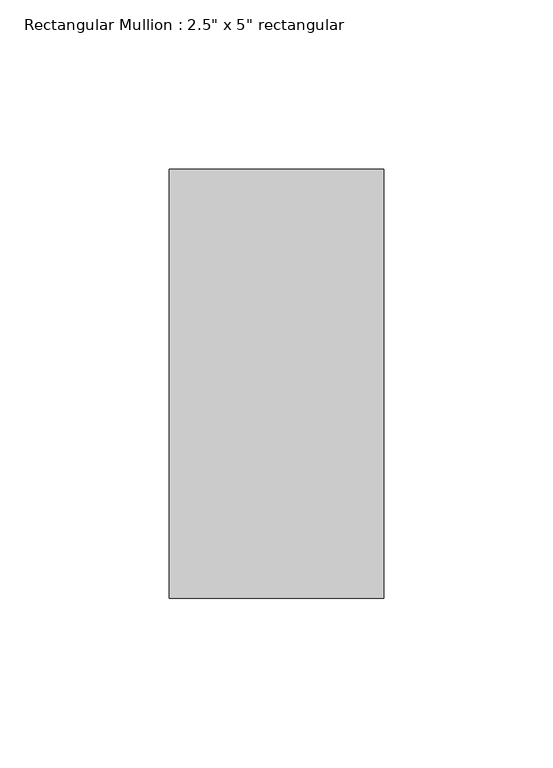
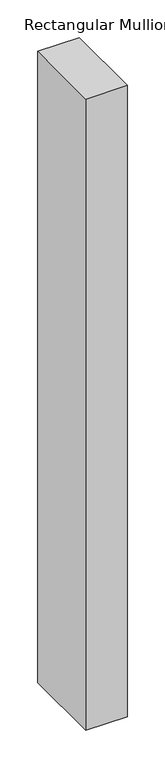
"""IFC4 building model written with IfcOpenShell, lengths in millimetres: member geometry."""

from ifc_helpers import new_model, si_unit, frame, origin, place, context, project, spatial, polyline, outline, extrude, source, transform, mapped, element, save


def member_0bcad3a7(model_context):
    return source(origin(), model_context, "Body", "SweptSolid", [
        extrude(outline(polyline([(0.0, 63.5), (0.0, -63.5), (-63.5, -63.5), (-63.5, 63.5), (0.0, 63.5)])), frame((0.0, 0.0, -1021.4266912), z_axis=(0.0, 0.0, 1.0), x_axis=(1.0, 0.0, 0.0)), (0.0, 0.0, 1.0), 1021.4266912),
    ])


if __name__ == "__main__":
    model = new_model("IFC4")
    model_context = context("Model", 3, world=origin())
    ifc_project = project(units=[si_unit("LENGTHUNIT", "METRE", prefix="MILLI")], contexts=[model_context])
    site = spatial("IfcSite", under=ifc_project)
    building = spatial("IfcBuilding", under=site)
    placement = place(None, origin())
    member_shape = member_0bcad3a7(model_context)
    element("IfcMember", 1, ObjectType="Rectangular Mullion : 2.5\" x 5\" rectangular", at=placement, inside=building, context=model_context, shape_type="MappedRepresentation", body=[
        mapped(member_shape, transform((0.0, 0.0, 0.0), x_axis=(1.0, 0.0, 0.0), y_axis=(0.0, 1.0, 0.0), z_axis=(0.0, 0.0, 1.0))),
    ])
    save(model, "model.ifc")

# Revit data of these elements
# Type "Rectangular Mullion : 2.5\" x 5\" rectangular"
#   built-in parameter 1007304 = 0.416667 (stored number, unit not read)
#   built-in parameter 1007301 = 0.104167 (stored number, unit not read)
#   built-in parameter 1007300 = 0.104167 (stored number, unit not read)
# Element 1 (IfcMember, "Rectangular Mullion : 2.5\" x 5\" rectangular")
#   Materials on its faces: "Aluminum"
# Materials
#   "Aluminum": class "Metal", colour RGB 247 247 247, transparency 0, Description = "Aluminum 6061", Cost = 0
